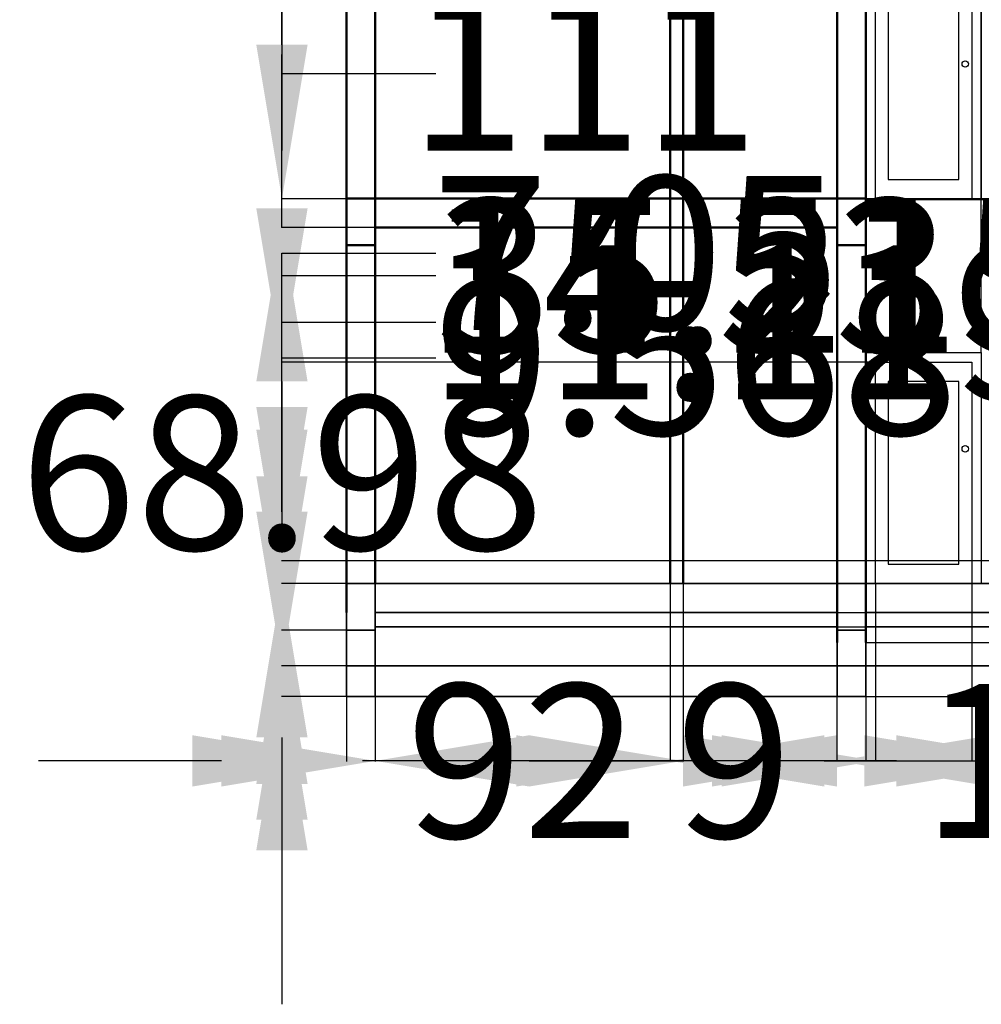
# Model space of a CAD drawing. Units: inches. Extents: x 131 to 858, y -65 to 554.
# Tile 1 of 4: x 131 to 431, y -65 to 242. Entities that reach past the tile are written whole.
import ezdxf

# ---------------------------------------------------------------- set-up
doc = ezdxf.new("R2010")
doc.units = ezdxf.units.IN
doc.header["$MEASUREMENT"] = 0
for name, color, linetype, lineweight in [('A-ANNO-DIMS', 2, 'Continuous', 18), ('A-DOOR', 4, 'Continuous', 25), ('A-SECT', 7, 'Continuous', 50), ('S-FNDN', 1, 'Continuous', 35)]:
    doc.layers.add(name, color=color, linetype=linetype, lineweight=lineweight)
doc.styles.get("Standard").update_dxf_attribs({"font": 'arial.ttf'})
doc.dimstyles.get("Standard").update_dxf_attribs({"dimtxt": 48, "dimasz": 48, "dimexe": 0.18, "dimexo": 0.0625, "dimgap": 0.09, "dimtad": 0, "dimtih": 1, "dimtoh": 1, "dimdec": 0, "dimrnd": 72, "dimzin": 0, "dimdsep": 46, "dimlunit": 3, "dimtxsty": 'Standard', "dimcen": 0.09, "dimadec": 0, "dimazin": 0, "dimtfac": 1, "dimtdec": 0, "dimtofl": 0, "dimtmove": 0, "dimatfit": 3, "dimfxl": 1, "dimtolj": 1, "dimtzin": 0, "dimarcsym": 0})

# ---------------------------------------------------------------- blocks, each defined once
blk = doc.blocks.new('*U3')
blk.add_lwpolyline([(3.12, 0.01), (0.12, 0.01), (0.12, 72.01), (36.12, 72.01), (36.12, 0.01), (33.12, 0.01)])
for points in [[(33.12, 68.99), (33.12, 0.01), (3.12, 0.01), (3.12, 68.99)], [(29.12, 6.01), (29.12, 62.99), (7.12, 62.99), (7.12, 6.01)]]:
    blk.add_lwpolyline(points, close=True)
blk.add_circle((31.12, 42.01), 1)
blk = doc.blocks.new('*D6')
at = {"layer": 'A-ANNO-DIMS', "color": 0, "lineweight": -2, "transparency": 16777216}
for p, q in [((242.01, 177.49), (242.01, 11.06)), ((233.01, 171.97), (233.01, 11.06)), ((185.01, 11.24), (137.01, 11.24)), ((290.01, 11.24), (338.01, 11.24))]:
    blk.add_line(p, q, dxfattribs=at)
at = {"layer": 'A-ANNO-DIMS', "color": 0, "transparency": 16777216}
for points in [[(185.01, 19.24), (185.01, 3.24), (233.01, 11.24)], [(290.01, 19.24), (290.01, 3.24), (242.01, 11.24)]]:
    blk.add_solid(points, dxfattribs=at)
at = {"layer": 'Defpoints', "color": 0, "transparency": 16777216}
for p in [(242.01, 177.55), (233.01, 172.03), (242.01, 11.24)]:
    blk.add_point(p, dxfattribs=at)
at = {"layer": 'A-ANNO-DIMS', "color": 0, "transparency": 16777216, "insert": (353.89, 11.24), "char_height": 48, "attachment_point": 5}
blk.add_mtext('\\A1;9', dxfattribs=at)
blk = doc.blocks.new('*D7')
at = {"layer": 'A-ANNO-DIMS', "color": 0, "lineweight": -2, "transparency": 16777216}
for p, q in [((334.014446, 66.488918), (334.014446, 11.056024)), ((242.014446, 31.273524), (242.014446, 11.056024)), ((194.014446, 11.236024), (146.014446, 11.236024)), ((382.014446, 11.236024), (430.014446, 11.236024))]:
    blk.add_line(p, q, dxfattribs=at)
at = {"layer": 'A-ANNO-DIMS', "color": 0, "transparency": 16777216}
for points in [[(194.014446, 19.236024), (194.014446, 3.236024), (242.014446, 11.236024)], [(382.014446, 19.236024), (382.014446, 3.236024), (334.014446, 11.236024)]]:
    blk.add_solid(points, dxfattribs=at)
at = {"layer": 'Defpoints', "color": 0, "transparency": 16777216}
for p in [(334.014446, 66.551418), (242.014446, 31.336024), (334.014446, 11.236024)]:
    blk.add_point(p, dxfattribs=at)
at = {"layer": 'A-ANNO-DIMS', "color": 0, "transparency": 16777216, "insert": (288.014446, 11.236024), "char_height": 48, "attachment_point": 5}
blk.add_mtext('\\A1;92', dxfattribs=at)
blk = doc.blocks.new('*D8')
at = {"layer": 'A-ANNO-DIMS', "color": 0, "lineweight": -2, "transparency": 16777216}
for p, q in [((334.01, 66.49), (334.01, 11.06)), ((338.01, 66.49), (338.01, 11.06)), ((286.01, 11.24), (238.01, 11.24)), ((386.01, 11.24), (434.01, 11.24))]:
    blk.add_line(p, q, dxfattribs=at)
at = {"layer": 'A-ANNO-DIMS', "color": 0, "transparency": 16777216}
for points in [[(286.01, 19.24), (286.01, 3.24), (334.01, 11.24)], [(386.01, 19.24), (386.01, 3.24), (338.01, 11.24)]]:
    blk.add_solid(points, dxfattribs=at)
at = {"layer": 'Defpoints', "color": 0, "transparency": 16777216}
for p in [(334.01, 66.55), (338.01, 66.55), (338.01, 11.24)]:
    blk.add_point(p, dxfattribs=at)
at = {"layer": 'A-ANNO-DIMS', "color": 0, "transparency": 16777216, "insert": (450.7, 11.24), "char_height": 48, "attachment_point": 5}
blk.add_mtext('\\A1;4', dxfattribs=at)
blk = doc.blocks.new('*D9')
at = {"layer": 'A-ANNO-DIMS', "color": 0, "lineweight": -2, "transparency": 16777216}
for p, q in [((338.01, 66.49), (338.01, 11.06)), ((386.01, 31.27), (386.01, 11.06)), ((290.01, 11.24), (242.01, 11.24)), ((434.01, 11.24), (482.01, 11.24))]:
    blk.add_line(p, q, dxfattribs=at)
at = {"layer": 'A-ANNO-DIMS', "color": 0, "transparency": 16777216}
for points in [[(290.01, 19.24), (290.01, 3.24), (338.01, 11.24)], [(434.01, 19.24), (434.01, 3.24), (386.01, 11.24)]]:
    blk.add_solid(points, dxfattribs=at)
at = {"layer": 'Defpoints', "color": 0, "transparency": 16777216}
for p in [(338.01, 66.55), (386.01, 31.34), (386.01, 11.24)]:
    blk.add_point(p, dxfattribs=at)
at = {"layer": 'A-ANNO-DIMS', "color": 0, "transparency": 16777216, "insert": (517.5, 11.24), "char_height": 48, "attachment_point": 5}
blk.add_mtext('\\A1;48', dxfattribs=at)
blk = doc.blocks.new('*D10')
at = {"layer": 'A-ANNO-DIMS', "color": 0, "lineweight": -2, "transparency": 16777216}
for p, q in [((386.01, 31.27), (386.01, 11.06)), ((395.01, 31.27), (395.01, 11.06)), ((338.01, 11.24), (290.01, 11.24)), ((443.01, 11.24), (491.01, 11.24))]:
    blk.add_line(p, q, dxfattribs=at)
at = {"layer": 'A-ANNO-DIMS', "color": 0, "transparency": 16777216}
for points in [[(338.01, 19.24), (338.01, 3.24), (386.01, 11.24)], [(443.01, 19.24), (443.01, 3.24), (395.01, 11.24)]]:
    blk.add_solid(points, dxfattribs=at)
at = {"layer": 'Defpoints', "color": 0, "transparency": 16777216}
for p in [(386.01, 31.34), (395.01, 31.34), (395.01, 11.24)]:
    blk.add_point(p, dxfattribs=at)
at = {"layer": 'A-ANNO-DIMS', "color": 0, "transparency": 16777216, "insert": (506.89, 11.24), "char_height": 48, "attachment_point": 5}
blk.add_mtext('\\A1;9', dxfattribs=at)
blk = doc.blocks.new('*D11')
at = {"layer": 'A-ANNO-DIMS', "color": 0, "lineweight": -2, "transparency": 16777216}
for p, q in [((395.014446, 31.273524), (395.014446, 11.056024)), ((539.014446, 31.273524), (539.014446, 11.056024)), ((347.014446, 11.236024), (299.014446, 11.236024)), ((587.014446, 11.236024), (635.014446, 11.236024))]:
    blk.add_line(p, q, dxfattribs=at)
at = {"layer": 'A-ANNO-DIMS', "color": 0, "transparency": 16777216}
for points in [[(347.014446, 19.236024), (347.014446, 3.236024), (395.014446, 11.236024)], [(587.014446, 19.236024), (587.014446, 3.236024), (539.014446, 11.236024)]]:
    blk.add_solid(points, dxfattribs=at)
at = {"layer": 'Defpoints', "color": 0, "transparency": 16777216}
for p in [(395.014446, 31.336024), (539.014446, 31.336024), (539.014446, 11.236024)]:
    blk.add_point(p, dxfattribs=at)
at = {"layer": 'A-ANNO-DIMS', "color": 0, "transparency": 16777216, "insert": (467.014446, 11.236024), "char_height": 48, "attachment_point": 5}
blk.add_mtext('\\A1;144', dxfattribs=at)
blk = doc.blocks.new('*D14')
at = {"layer": 'A-ANNO-DIMS', "color": 0, "lineweight": -2, "transparency": 16777216}
for p, q in [((592.11, 426.55), (612.82, 426.55)), ((612.64, 378.55), (612.64, 253.56)), ((612.64, 79.34), (612.64, 204.33)), ((233.08, 31.34), (612.82, 31.34))]:
    blk.add_line(p, q, dxfattribs=at)
at = {"layer": 'A-ANNO-DIMS', "color": 0, "transparency": 16777216}
for points in [[(604.64, 378.55), (620.64, 378.55), (612.64, 426.55)], [(604.64, 79.34), (620.64, 79.34), (612.64, 31.34)]]:
    blk.add_solid(points, dxfattribs=at)
at = {"layer": 'Defpoints', "color": 0, "transparency": 16777216}
for p in [(592.04, 426.55), (612.64, 426.55), (233.01, 31.34)]:
    blk.add_point(p, dxfattribs=at)
at = {"layer": 'A-ANNO-DIMS', "color": 0, "transparency": 16777216, "insert": (612.64, 228.94), "char_height": 48, "attachment_point": 5}
blk.add_mtext('\\A1;395.2', dxfattribs=at)
blk = doc.blocks.new('*D15')
at = {"layer": 'A-ANNO-DIMS', "color": 0, "lineweight": -2, "transparency": 16777216}
for p, q in [((212.91, 114.55), (212.91, 162.55)), ((212.91, 162.55), (260.91, 162.55)), ((385.95, 66.55), (212.73, 66.55)), ((385.95, 31.34), (212.73, 31.34)), ((212.91, -16.66), (212.91, -64.66))]:
    blk.add_line(p, q, dxfattribs=at)
at = {"layer": 'A-ANNO-DIMS', "color": 0, "transparency": 16777216}
for points in [[(204.91, 114.55), (220.91, 114.55), (212.91, 66.55)], [(204.91, -16.66), (220.91, -16.66), (212.91, 31.34)]]:
    blk.add_solid(points, dxfattribs=at)
at = {"layer": 'Defpoints', "color": 0, "transparency": 16777216}
for p in [(212.91, 66.55), (386.01, 66.55), (386.01, 31.34)]:
    blk.add_point(p, dxfattribs=at)
at = {"layer": 'A-ANNO-DIMS', "color": 0, "transparency": 16777216, "insert": (360.8, 162.55), "char_height": 48, "attachment_point": 5}
blk.add_mtext('\\A1;35.215', dxfattribs=at)
blk = doc.blocks.new('*D16')
at = {"layer": 'A-ANNO-DIMS', "color": 0, "lineweight": -2, "transparency": 16777216}
for p, q in [((212.91, 88.9), (212.91, 136.9)), ((212.91, 136.9), (260.91, 136.9)), ((232.95, 40.9), (212.73, 40.9)), ((232.95, 31.34), (212.73, 31.34)), ((212.91, -16.66), (212.91, -64.66))]:
    blk.add_line(p, q, dxfattribs=at)
at = {"layer": 'A-ANNO-DIMS', "color": 0, "transparency": 16777216}
for points in [[(204.91, 88.9), (220.91, 88.9), (212.91, 40.9)], [(204.91, -16.66), (220.91, -16.66), (212.91, 31.34)]]:
    blk.add_solid(points, dxfattribs=at)
at = {"layer": 'Defpoints', "color": 0, "transparency": 16777216}
for p in [(212.91, 40.9), (233.01, 40.9), (233.01, 31.34)]:
    blk.add_point(p, dxfattribs=at)
at = {"layer": 'A-ANNO-DIMS', "color": 0, "transparency": 16777216, "insert": (342.04, 136.9), "char_height": 48, "attachment_point": 5}
blk.add_mtext('\\A1;9.568', dxfattribs=at)
blk = doc.blocks.new('*D17')
at = {"layer": 'A-ANNO-DIMS', "color": 0, "lineweight": -2, "transparency": 16777216}
for p, q in [((212.91, 100.02), (212.91, 148.02)), ((212.91, 148.02), (260.91, 148.02)), ((232.95, 52.02), (212.73, 52.02)), ((232.95, 40.9), (212.73, 40.9)), ((212.91, -7.1), (212.91, -55.1))]:
    blk.add_line(p, q, dxfattribs=at)
at = {"layer": 'A-ANNO-DIMS', "color": 0, "transparency": 16777216}
for points in [[(204.91, 100.02), (220.91, 100.02), (212.91, 52.02)], [(204.91, -7.1), (220.91, -7.1), (212.91, 40.9)]]:
    blk.add_solid(points, dxfattribs=at)
at = {"layer": 'Defpoints', "color": 0, "transparency": 16777216}
for p in [(212.91, 52.02), (233.01, 52.02), (233.01, 40.9)]:
    blk.add_point(p, dxfattribs=at)
at = {"layer": 'A-ANNO-DIMS', "color": 0, "transparency": 16777216, "insert": (358.43, 148.02), "char_height": 48, "attachment_point": 5}
blk.add_mtext('\\A1;11.119', dxfattribs=at)
blk = doc.blocks.new('*D18')
at = {"layer": 'A-ANNO-DIMS', "color": 0, "lineweight": -2, "transparency": 16777216}
for p, q in [((212.91, 114.55), (212.91, 162.55)), ((212.91, 162.55), (260.91, 162.55)), ((232.95, 66.55), (212.73, 66.55)), ((232.95, 52.02), (212.73, 52.02)), ((212.91, 4.02), (212.91, -43.98))]:
    blk.add_line(p, q, dxfattribs=at)
at = {"layer": 'A-ANNO-DIMS', "color": 0, "transparency": 16777216}
for points in [[(204.91, 114.55), (220.91, 114.55), (212.91, 66.55)], [(204.91, 4.02), (220.91, 4.02), (212.91, 52.02)]]:
    blk.add_solid(points, dxfattribs=at)
at = {"layer": 'Defpoints', "color": 0, "transparency": 16777216}
for p in [(212.91, 66.55), (233.01, 66.55), (233.01, 52.02)]:
    blk.add_point(p, dxfattribs=at)
at = {"layer": 'A-ANNO-DIMS', "color": 0, "transparency": 16777216, "insert": (339.73, 162.55), "char_height": 48, "attachment_point": 5}
blk.add_mtext('\\A1;14.53', dxfattribs=at)
blk = doc.blocks.new('*D19')
at = {"layer": 'A-ANNO-DIMS', "color": 0, "lineweight": -2, "transparency": 16777216}
for p, q in [((612.64, 105.55), (612.64, 153.55)), ((612.64, 153.55), (660.64, 153.55)), ((242.08, 57.55), (612.82, 57.55)), ((242.08, 53.09), (612.82, 53.09)), ((612.64, 5.09), (612.64, -42.91))]:
    blk.add_line(p, q, dxfattribs=at)
at = {"layer": 'A-ANNO-DIMS', "color": 0, "transparency": 16777216}
for points in [[(604.64, 105.55), (620.64, 105.55), (612.64, 57.55)], [(604.64, 5.09), (620.64, 5.09), (612.64, 53.09)]]:
    blk.add_solid(points, dxfattribs=at)
at = {"layer": 'Defpoints', "color": 0, "transparency": 16777216}
for p in [(242.01, 57.55), (612.64, 57.55), (242.01, 53.09)]:
    blk.add_point(p, dxfattribs=at)
at = {"layer": 'A-ANNO-DIMS', "color": 0, "transparency": 16777216, "insert": (742.86, 153.55), "char_height": 48, "attachment_point": 5}
blk.add_mtext('\\A1;4.465', dxfattribs=at)
blk = doc.blocks.new('*D20')
at = {"layer": 'A-ANNO-DIMS', "color": 0, "lineweight": -2, "transparency": 16777216}
for p, q in [((612.64, 114.55), (612.64, 162.55)), ((612.64, 162.55), (660.64, 162.55)), ((242.08, 66.55), (612.82, 66.55)), ((242.08, 57.55), (612.82, 57.55)), ((612.64, 9.55), (612.64, -38.45))]:
    blk.add_line(p, q, dxfattribs=at)
at = {"layer": 'A-ANNO-DIMS', "color": 0, "transparency": 16777216}
for points in [[(604.64, 114.55), (620.64, 114.55), (612.64, 66.55)], [(604.64, 9.55), (620.64, 9.55), (612.64, 57.55)]]:
    blk.add_solid(points, dxfattribs=at)
at = {"layer": 'Defpoints', "color": 0, "transparency": 16777216}
for p in [(242.01, 66.55), (612.64, 66.55), (242.01, 57.55)]:
    blk.add_point(p, dxfattribs=at)
at = {"layer": 'A-ANNO-DIMS', "color": 0, "transparency": 16777216, "insert": (676.51, 162.55), "char_height": 48, "attachment_point": 5}
blk.add_mtext('\\A1;9', dxfattribs=at)
blk = doc.blocks.new('*D21')
at = {"layer": 'A-ANNO-DIMS', "color": 0, "lineweight": -2, "transparency": 16777216}
for p, q in [((233.01, 31.27), (233.01, 11.06)), ((242.01, 31.27), (242.01, 11.06)), ((185.01, 11.24), (137.01, 11.24)), ((290.01, 11.24), (338.01, 11.24))]:
    blk.add_line(p, q, dxfattribs=at)
at = {"layer": 'A-ANNO-DIMS', "color": 0, "transparency": 16777216}
for points in [[(185.01, 19.24), (185.01, 3.24), (233.01, 11.24)], [(290.01, 19.24), (290.01, 3.24), (242.01, 11.24)]]:
    blk.add_solid(points, dxfattribs=at)
at = {"layer": 'Defpoints', "color": 0, "transparency": 16777216}
for p in [(233.01, 31.34), (242.01, 31.34), (242.01, 11.24)]:
    blk.add_point(p, dxfattribs=at)
at = {"layer": 'A-ANNO-DIMS', "color": 0, "transparency": 16777216, "insert": (353.89, 11.24), "char_height": 48, "attachment_point": 5}
blk.add_mtext('\\A1;9', dxfattribs=at)
blk = doc.blocks.new('*D22')
at = {"layer": 'A-ANNO-DIMS', "color": 0, "lineweight": -2, "transparency": 16777216}
for p, q in [((612.64, 114.55), (612.64, 162.55)), ((612.64, 162.55), (660.64, 162.55)), ((395.08, 66.55), (612.82, 66.55)), ((395.08, 48.13), (612.82, 48.13)), ((612.64, 0.13), (612.64, -47.87))]:
    blk.add_line(p, q, dxfattribs=at)
at = {"layer": 'A-ANNO-DIMS', "color": 0, "transparency": 16777216}
for points in [[(604.64, 114.55), (620.64, 114.55), (612.64, 66.55)], [(604.64, 0.13), (620.64, 0.13), (612.64, 48.13)]]:
    blk.add_solid(points, dxfattribs=at)
at = {"layer": 'Defpoints', "color": 0, "transparency": 16777216}
for p in [(395.01, 66.55), (612.64, 66.55), (395.01, 48.13)]:
    blk.add_point(p, dxfattribs=at)
at = {"layer": 'A-ANNO-DIMS', "color": 0, "transparency": 16777216, "insert": (758.11, 162.55), "char_height": 48, "attachment_point": 5}
blk.add_mtext('\\A1;18.417', dxfattribs=at)
blk = doc.blocks.new('*D23')
at = {"layer": 'A-ANNO-DIMS', "color": 0, "lineweight": -2, "transparency": 16777216}
for p, q in [((212.91, 177.55), (212.91, 225.55)), ((212.91, 225.55), (260.91, 225.55)), ((241.95, 177.55), (212.73, 177.55)), ((212.91, 114.55), (212.91, 129.55)), ((232.95, 66.55), (212.73, 66.55))]:
    blk.add_line(p, q, dxfattribs=at)
at = {"layer": 'A-ANNO-DIMS', "color": 0, "transparency": 16777216}
for points in [[(204.91, 129.55), (220.91, 129.55), (212.91, 177.55)], [(204.91, 114.55), (220.91, 114.55), (212.91, 66.55)]]:
    blk.add_solid(points, dxfattribs=at)
at = {"layer": 'Defpoints', "color": 0, "transparency": 16777216}
for p in [(212.91, 177.55), (242.01, 177.55), (233.01, 66.55)]:
    blk.add_point(p, dxfattribs=at)
at = {"layer": 'A-ANNO-DIMS', "color": 0, "transparency": 16777216, "insert": (307.14, 225.55), "char_height": 48, "attachment_point": 5}
blk.add_mtext('\\A1;111', dxfattribs=at)
blk = doc.blocks.new('*D24')
at = {"layer": 'A-ANNO-DIMS', "color": 0, "lineweight": -2, "transparency": 16777216}
for p, q in [((212.91, 234.55), (212.91, 282.55)), ((212.91, 282.55), (260.91, 282.55)), ((232.95, 186.55), (212.73, 186.55)), ((241.95, 177.55), (212.73, 177.55)), ((212.91, 129.55), (212.91, 81.55))]:
    blk.add_line(p, q, dxfattribs=at)
at = {"layer": 'A-ANNO-DIMS', "color": 0, "transparency": 16777216}
for points in [[(204.91, 234.55), (220.91, 234.55), (212.91, 186.55)], [(204.91, 129.55), (220.91, 129.55), (212.91, 177.55)]]:
    blk.add_solid(points, dxfattribs=at)
at = {"layer": 'Defpoints', "color": 0, "transparency": 16777216}
for p in [(212.91, 186.55), (233.01, 186.55), (242.01, 177.55)]:
    blk.add_point(p, dxfattribs=at)
at = {"layer": 'A-ANNO-DIMS', "color": 0, "transparency": 16777216, "insert": (276.79, 282.55), "char_height": 48, "attachment_point": 5}
blk.add_mtext('\\A1;9', dxfattribs=at)
blk = doc.blocks.new('*D25')
at = {"layer": 'A-ANNO-DIMS', "color": 0, "lineweight": -2, "transparency": 16777216}
for p, q in [((212.91, 297.55), (212.91, 345.55)), ((212.91, 345.55), (260.91, 345.55)), ((241.95, 297.55), (212.73, 297.55)), ((212.91, 234.55), (212.91, 249.55)), ((232.95, 186.55), (212.73, 186.55))]:
    blk.add_line(p, q, dxfattribs=at)
at = {"layer": 'A-ANNO-DIMS', "color": 0, "transparency": 16777216}
for points in [[(204.91, 249.55), (220.91, 249.55), (212.91, 297.55)], [(204.91, 234.55), (220.91, 234.55), (212.91, 186.55)]]:
    blk.add_solid(points, dxfattribs=at)
at = {"layer": 'Defpoints', "color": 0, "transparency": 16777216}
for p in [(212.91, 297.55), (242.01, 297.55), (233.01, 186.55)]:
    blk.add_point(p, dxfattribs=at)
at = {"layer": 'A-ANNO-DIMS', "color": 0, "transparency": 16777216, "insert": (307.14, 345.55), "char_height": 48, "attachment_point": 5}
blk.add_mtext('\\A1;111', dxfattribs=at)
blk = doc.blocks.new('*D26')
at = {"layer": 'A-ANNO-DIMS', "color": 0, "lineweight": -2, "transparency": 16777216}
for p, q in [((212.91, 354.55), (212.91, 402.55)), ((212.91, 402.55), (260.91, 402.55)), ((232.95, 306.55), (212.73, 306.55)), ((241.95, 297.55), (212.73, 297.55)), ((212.91, 249.55), (212.91, 201.55))]:
    blk.add_line(p, q, dxfattribs=at)
at = {"layer": 'A-ANNO-DIMS', "color": 0, "transparency": 16777216}
for points in [[(204.91, 354.55), (220.91, 354.55), (212.91, 306.55)], [(204.91, 249.55), (220.91, 249.55), (212.91, 297.55)]]:
    blk.add_solid(points, dxfattribs=at)
at = {"layer": 'Defpoints', "color": 0, "transparency": 16777216}
for p in [(212.91, 306.55), (233.01, 306.55), (242.01, 297.55)]:
    blk.add_point(p, dxfattribs=at)
at = {"layer": 'A-ANNO-DIMS', "color": 0, "transparency": 16777216, "insert": (276.79, 402.55), "char_height": 48, "attachment_point": 5}
blk.add_mtext('\\A1;9', dxfattribs=at)
blk = doc.blocks.new('*D27')
at = {"layer": 'A-ANNO-DIMS', "color": 0, "lineweight": -2, "transparency": 16777216}
for p, q in [((212.91, 402.55), (212.91, 450.55)), ((212.91, 450.55), (260.91, 450.55)), ((232.95, 354.55), (212.73, 354.55)), ((232.95, 306.55), (212.73, 306.55)), ((212.91, 258.55), (212.91, 210.55))]:
    blk.add_line(p, q, dxfattribs=at)
at = {"layer": 'A-ANNO-DIMS', "color": 0, "transparency": 16777216}
for points in [[(204.91, 402.55), (220.91, 402.55), (212.91, 354.55)], [(204.91, 258.55), (220.91, 258.55), (212.91, 306.55)]]:
    blk.add_solid(points, dxfattribs=at)
at = {"layer": 'Defpoints', "color": 0, "transparency": 16777216}
for p in [(212.91, 354.55), (233.01, 354.55), (233.01, 306.55)]:
    blk.add_point(p, dxfattribs=at)
at = {"layer": 'A-ANNO-DIMS', "color": 0, "transparency": 16777216, "insert": (296.4, 450.55), "char_height": 48, "attachment_point": 5}
blk.add_mtext('\\A1;48', dxfattribs=at)
blk = doc.blocks.new('*D32')
at = {"layer": 'A-ANNO-DIMS', "color": 0, "lineweight": -2, "transparency": 16777216}
for p, q in [((347.01, 446.65), (299.01, 446.65)), ((395.01, 138.61), (395.01, 446.83)), ((431.01, 138.61), (431.01, 446.83)), ((479.01, 446.65), (527.01, 446.65))]:
    blk.add_line(p, q, dxfattribs=at)
at = {"layer": 'A-ANNO-DIMS', "color": 0, "transparency": 16777216}
for points in [[(347.01, 454.65), (347.01, 438.65), (395.01, 446.65)], [(479.01, 454.65), (479.01, 438.65), (431.01, 446.65)]]:
    blk.add_solid(points, dxfattribs=at)
at = {"layer": 'Defpoints', "color": 0, "transparency": 16777216}
for p in [(431.01, 446.65), (395.01, 138.55), (431.01, 138.55)]:
    blk.add_point(p, dxfattribs=at)
at = {"layer": 'A-ANNO-DIMS', "color": 0, "transparency": 16777216, "insert": (561.45, 446.65), "char_height": 48, "attachment_point": 5}
blk.add_mtext('\\A1;36', dxfattribs=at)
blk = doc.blocks.new('*D34')
at = {"layer": 'A-ANNO-DIMS', "color": 0, "lineweight": -2, "transparency": 16777216}
for p, q in [((398.01, 66.49), (398.01, 11.06)), ((428.01, 66.49), (428.01, 11.06)), ((350.01, 11.24), (302.01, 11.24)), ((476.01, 11.24), (524.01, 11.24))]:
    blk.add_line(p, q, dxfattribs=at)
at = {"layer": 'A-ANNO-DIMS', "color": 0, "transparency": 16777216}
for points in [[(350.01, 19.24), (350.01, 3.24), (398.01, 11.24)], [(476.01, 19.24), (476.01, 3.24), (428.01, 11.24)]]:
    blk.add_solid(points, dxfattribs=at)
at = {"layer": 'Defpoints', "color": 0, "transparency": 16777216}
for p in [(398.01, 66.55), (428.01, 66.55), (428.01, 11.24)]:
    blk.add_point(p, dxfattribs=at)
at = {"layer": 'A-ANNO-DIMS', "color": 0, "transparency": 16777216, "insert": (558.39, 11.24), "char_height": 48, "attachment_point": 5}
blk.add_mtext('\\A1;30', dxfattribs=at)
blk = doc.blocks.new('*D35')
at = {"layer": 'A-ANNO-DIMS', "color": 0, "lineweight": -2, "transparency": 16777216}
for p, q in [((212.91, 183.53), (212.91, 231.53)), ((397.95, 135.53), (212.73, 135.53)), ((397.95, 66.55), (212.73, 66.55)), ((212.91, 18.55), (212.91, -29.45))]:
    blk.add_line(p, q, dxfattribs=at)
at = {"layer": 'A-ANNO-DIMS', "color": 0, "transparency": 16777216}
for points in [[(204.91, 183.53), (220.91, 183.53), (212.91, 135.53)], [(204.91, 18.55), (220.91, 18.55), (212.91, 66.55)]]:
    blk.add_solid(points, dxfattribs=at)
at = {"layer": 'Defpoints', "color": 0, "transparency": 16777216}
for p in [(212.91, 135.53), (398.01, 135.53), (398.01, 66.55)]:
    blk.add_point(p, dxfattribs=at)
at = {"layer": 'A-ANNO-DIMS', "color": 0, "transparency": 16777216, "insert": (212.91, 101.04), "char_height": 48, "attachment_point": 5}
blk.add_mtext('\\A1;68.98', dxfattribs=at)
blk = doc.blocks.new('*D36')
at = {"layer": 'A-ANNO-DIMS', "color": 0, "lineweight": -2, "transparency": 16777216}
for p, q in [((452.53, 73.54), (452.53, 11.06)), ((442.52, 66.49), (442.52, 11.06)), ((394.52, 11.24), (346.52, 11.24)), ((500.53, 11.24), (548.53, 11.24))]:
    blk.add_line(p, q, dxfattribs=at)
at = {"layer": 'A-ANNO-DIMS', "color": 0, "transparency": 16777216}
for points in [[(394.52, 19.24), (394.52, 3.24), (442.52, 11.24)], [(500.53, 19.24), (500.53, 3.24), (452.53, 11.24)]]:
    blk.add_solid(points, dxfattribs=at)
at = {"layer": 'Defpoints', "color": 0, "transparency": 16777216}
for p in [(452.53, 73.6), (442.52, 66.55), (452.53, 11.24)]:
    blk.add_point(p, dxfattribs=at)
at = {"layer": 'A-ANNO-DIMS', "color": 0, "transparency": 16777216, "insert": (646, 11.24), "char_height": 48, "attachment_point": 5}
blk.add_mtext('\\A1;10.013', dxfattribs=at)
blk = doc.blocks.new('*D37')
at = {"layer": 'A-ANNO-DIMS', "color": 0, "lineweight": -2, "transparency": 16777216}
for p, q in [((544.04, 126.29), (544.04, 11.06)), ((452.53, 73.54), (452.53, 11.06)), ((404.53, 11.24), (356.53, 11.24)), ((592.04, 11.24), (640.04, 11.24))]:
    blk.add_line(p, q, dxfattribs=at)
at = {"layer": 'A-ANNO-DIMS', "color": 0, "transparency": 16777216}
for points in [[(404.53, 19.24), (404.53, 3.24), (452.53, 11.24)], [(592.04, 19.24), (592.04, 3.24), (544.04, 11.24)]]:
    blk.add_solid(points, dxfattribs=at)
at = {"layer": 'Defpoints', "color": 0, "transparency": 16777216}
for p in [(544.04, 126.36), (452.53, 73.6), (544.04, 11.24)]:
    blk.add_point(p, dxfattribs=at)
at = {"layer": 'A-ANNO-DIMS', "color": 0, "transparency": 16777216, "insert": (716.49, 11.24), "char_height": 48, "attachment_point": 5}
blk.add_mtext('\\A1;91.51', dxfattribs=at)
blk = doc.blocks.new('*D40')
at = {"layer": 'A-ANNO-DIMS', "color": 0, "lineweight": -2, "transparency": 16777216}
for p, q in [((212.91, 121.6), (212.91, 169.6)), ((212.91, 169.6), (260.91, 169.6)), ((442.46, 73.6), (212.73, 73.6)), ((442.46, 66.55), (212.73, 66.55)), ((212.91, 18.55), (212.91, -29.45))]:
    blk.add_line(p, q, dxfattribs=at)
at = {"layer": 'A-ANNO-DIMS', "color": 0, "transparency": 16777216}
for points in [[(204.91, 121.6), (220.91, 121.6), (212.91, 73.6)], [(204.91, 18.55), (220.91, 18.55), (212.91, 66.55)]]:
    blk.add_solid(points, dxfattribs=at)
at = {"layer": 'Defpoints', "color": 0, "transparency": 16777216}
for p in [(212.91, 73.6), (442.52, 73.6), (442.52, 66.55)]:
    blk.add_point(p, dxfattribs=at)
at = {"layer": 'A-ANNO-DIMS', "color": 0, "transparency": 16777216, "insert": (323.33, 169.6), "char_height": 48, "attachment_point": 5}
blk.add_mtext('\\A1;7.05', dxfattribs=at)

msp = doc.modelspace()

# ---------------------------------------------------------------- linework, layer by layer
at = {"layer": 'A-SECT'}
for p, q in [((395.0144, 48.1342), (395.0144, 366.3568)), ((386.0144, 48.1342), (386.0144, 354.5514)), ((233.0144, 306.5514), (233.0144, 57.5514)), ((242.0144, 306.5514), (242.0144, 66.5514)), ((334.0144, 306.5514), (334.0144, 66.5514)), ((338.0144, 306.5514), (338.0144, 66.5514)), ((386.0144, 306.5514), (386.0144, 66.5514)), ((395.0144, 306.5514), (395.0144, 57.5514)), ((233.0144, 172.0345), (233.0144, 186.5514)), ((233.0144, 186.5514), (242.0144, 186.5514)), ((242.0144, 186.5514), (386.0144, 186.5514)), ((242.0144, 186.5514), (386.0144, 186.5514)), ((242.0144, 186.5514), (242.0144, 177.5514)), ((386.0144, 172.0345), (386.0144, 186.5514)), ((386.0144, 186.5514), (395.0144, 186.5514)), ((395.0144, 186.5514), (395.0144, 177.5514)), ((395.0144, 186.3568), (443.0144, 186.3568)), ((395.0144, 186.3568), (395.0144, 48.1342)), ((242.0144, 177.5514), (386.0144, 177.5514)), ((242.0144, 172.0345), (233.0144, 172.0345)), ((395.0144, 172.0345), (386.0144, 172.0345))]:
    msp.add_line(p, q, dxfattribs=at)
at = {"layer": 'S-FNDN'}
for p, q in [((242.0144, 66.5514), (233.0144, 66.5514)), ((242.0144, 66.5514), (386.0144, 66.5514)), ((242.0144, 66.5514), (242.0144, 57.5514)), ((386.0144, 66.5514), (395.0144, 66.5514)), ((395.0144, 66.5514), (386.0144, 66.5514)), ((386.0144, 66.5514), (386.0144, 57.5514)), ((395.0144, 66.5514), (386.0144, 66.5514)), ((442.5179, 66.5514), (386.0144, 66.5514)), ((395.0144, 66.5514), (548.0144, 66.5514)), ((395.0144, 66.5514), (395.0144, 57.5514)), ((233.0144, 31.336), (233.0144, 57.5514)), ((242.0144, 57.5514), (386.0144, 57.5514)), ((242.0144, 57.5514), (242.0144, 31.336)), ((386.0144, 31.336), (386.0144, 57.5514)), ((395.0144, 57.5514), (539.0144, 57.5514)), ((395.0144, 57.5514), (395.0144, 31.336)), ((242.0144, 53.0868), (386.0144, 53.0868)), ((395.0144, 53.0868), (539.0144, 53.0868)), ((233.0144, 52.0226), (242.0144, 52.0226)), ((386.0144, 52.0226), (395.0144, 52.0226)), ((386.0144, 52.0226), (395.0144, 52.0226)), ((233.0144, 40.9038), (548.0144, 40.9038)), ((233.0144, 31.336), (242.0144, 31.336)), ((386.0144, 31.336), (395.0144, 31.336))]:
    msp.add_line(p, q, dxfattribs=at)

# ---------------------------------------------------------------- block references
at = {"layer": 'A-DOOR'}
for p in [(394.8907, 186.5387), (394.8907, 66.5387)]:
    msp.add_blockref('*U3', p, dxfattribs=at)

# ---------------------------------------------------------------- dimensions: what is measured, and where the dimension line sits
at = {"layer": 'A-ANNO-DIMS'}
for base, p1, p2, override, picture, middle in [((212.9144, 354.5514), (233.0144, 306.5514), (233.0144, 354.5514), {"dimdec": 0, "dimlfac": 1, "dimrnd": 0, "dimzin": 0, "dimdsep": 46, "dimlunit": 2}, '*D27', (296.3987, 450.5514)), ((212.9144, 306.5514), (242.0144, 297.5514), (233.0144, 306.5514), {"dimdec": 0, "dimlfac": 1, "dimrnd": 0, "dimzin": 0, "dimdsep": 46, "dimlunit": 2}, '*D26', (276.7862, 402.5514)), ((612.64, 426.5514), (233.0144, 31.336), (592.0434, 426.5514), {"dimdec": 1, "dimlfac": 1, "dimrnd": 0, "dimzin": 0, "dimdsep": 46, "dimlunit": 2}, '*D14', (612.64, 228.9437)), ((212.9144, 297.5514), (233.0144, 186.5514), (242.0144, 297.5514), {"dimdec": 0, "dimlfac": 1, "dimrnd": 0, "dimzin": 0, "dimdsep": 46, "dimlunit": 2}, '*D25', (307.1381, 345.5514)), ((212.9144, 186.5514), (242.0144, 177.5514), (233.0144, 186.5514), {"dimdec": 0, "dimlfac": 1, "dimrnd": 0, "dimzin": 0, "dimdsep": 46, "dimlunit": 2}, '*D24', (276.7862, 282.5514)), ((212.9144, 177.5514), (233.0144, 66.5514), (242.0144, 177.5514), {"dimdec": 0, "dimlfac": 1, "dimrnd": 0, "dimzin": 0, "dimdsep": 46, "dimlunit": 2}, '*D23', (307.1381, 225.5514)), ((212.9144, 135.5284), (398.0144, 66.5514), (398.0144, 135.5284), {"dimdec": 2, "dimlfac": 1, "dimrnd": 0, "dimzin": 0, "dimdsep": 46, "dimlunit": 2}, '*D35', (212.9144, 101.0399)), ((212.9144, 73.6016), (442.5179, 66.5514), (442.5179, 73.6016), {"dimdec": 2, "dimlfac": 1, "dimrnd": 0, "dimzin": 0, "dimdsep": 46, "dimlunit": 2}, '*D40', (323.3291, 169.6016)), ((212.9144, 66.5514), (386.0144, 31.336), (386.0144, 66.5514), {"dimdec": 3, "dimlfac": 1, "dimrnd": 0, "dimzin": 0, "dimdsep": 46, "dimlunit": 2}, '*D15', (360.8025, 162.5514)), ((212.9144, 66.5514), (233.0144, 52.0226), (233.0144, 66.5514), {"dimdec": 2, "dimlfac": 1, "dimrnd": 0, "dimzin": 0, "dimdsep": 46, "dimlunit": 2}, '*D18', (339.733, 162.5514)), ((612.64, 66.5514), (242.0144, 57.5514), (242.0144, 66.5514), {"dimdec": 0, "dimlfac": 1, "dimrnd": 0, "dimzin": 0, "dimdsep": 46, "dimlunit": 2}, '*D20', (676.5117, 162.5514)), ((612.64, 66.5514), (395.0144, 48.1342), (395.0144, 66.5514), {"dimdec": 3, "dimlfac": 1, "dimrnd": 0, "dimzin": 0, "dimdsep": 46, "dimlunit": 2}, '*D22', (758.1051, 162.5514)), ((612.64, 57.5514), (242.0144, 53.0868), (242.0144, 57.5514), {"dimdec": 3, "dimlfac": 1, "dimrnd": 0, "dimzin": 0, "dimdsep": 46, "dimlunit": 2}, '*D19', (742.8637, 153.5514)), ((212.9144, 52.0226), (233.0144, 40.9038), (233.0144, 52.0226), {"dimdec": 3, "dimlfac": 1, "dimrnd": 0, "dimzin": 0, "dimdsep": 46, "dimlunit": 2}, '*D17', (358.4287, 148.0226)), ((212.9144, 40.9038), (233.0144, 31.336), (233.0144, 40.9038), {"dimdec": 3, "dimlfac": 1, "dimrnd": 0, "dimzin": 0, "dimdsep": 46, "dimlunit": 2}, '*D16', (342.0413, 136.9038))]:
    dim = msp.add_linear_dim(base=base, p1=p1, p2=p2, angle=90, dimstyle='Standard', override=override, dxfattribs=at)
    dim.commit()
    dim.dimension.update_dxf_attribs({"geometry": picture, "text_midpoint": middle})
for base, p1, p2, override, picture, middle in [((431.0144, 446.6514), (395.0144, 138.5514), (431.0144, 138.5514), {"dimdec": 0, "dimlfac": 1, "dimrnd": 0, "dimzin": 0, "dimdsep": 46, "dimlunit": 2}, '*D32', (561.451, 446.6514)), ((242.0144, 11.236), (233.0144, 172.0345), (242.0144, 177.5514), {"dimdec": 0, "dimlfac": 1, "dimrnd": 0, "dimzin": 0, "dimdsep": 46, "dimlunit": 2}, '*D6', (353.8862, 11.236)), ((544.0434, 11.236), (452.5306, 73.6016), (544.0434, 126.3568), {"dimdec": 2, "dimlfac": 1, "dimrnd": 0, "dimzin": 0, "dimdsep": 46, "dimlunit": 2}, '*D37', (716.4881, 11.236)), ((452.5306, 11.236), (442.5179, 66.5514), (452.5306, 73.6016), {"dimdec": 3, "dimlfac": 1, "dimrnd": 0, "dimzin": 0, "dimdsep": 46, "dimlunit": 2}, '*D36', (645.9958, 11.236)), ((334.0144, 11.236), (242.0144, 31.336), (334.0144, 66.5514), {"dimdec": 0, "dimlfac": 1, "dimrnd": 0, "dimzin": 0, "dimdsep": 46, "dimlunit": 2}, '*D7', (288.0144, 11.236)), ((338.0144, 11.236), (334.0144, 66.5514), (338.0144, 66.5514), {"dimdec": 0, "dimlfac": 1, "dimrnd": 0, "dimzin": 0, "dimdsep": 46, "dimlunit": 2}, '*D8', (450.7047, 11.236)), ((386.0144, 11.236), (338.0144, 66.5514), (386.0144, 31.336), {"dimdec": 0, "dimlfac": 1, "dimrnd": 0, "dimzin": 0, "dimdsep": 46, "dimlunit": 2}, '*D9', (517.4987, 11.236)), ((428.0144, 11.236), (398.0144, 66.5514), (428.0144, 66.5514), {"dimdec": 0, "dimlfac": 1, "dimrnd": 0, "dimzin": 0, "dimdsep": 46, "dimlunit": 2}, '*D34', (558.3855, 11.236)), ((242.0144, 11.236), (233.0144, 31.336), (242.0144, 31.336), {"dimdec": 0, "dimlfac": 1, "dimrnd": 0, "dimzin": 0, "dimdsep": 46, "dimlunit": 2}, '*D21', (353.8862, 11.236)), ((395.0144, 11.236), (386.0144, 31.336), (395.0144, 31.336), {"dimdec": 0, "dimlfac": 1, "dimrnd": 0, "dimzin": 0, "dimdsep": 46, "dimlunit": 2}, '*D10', (506.8862, 11.236)), ((539.0144, 11.236), (395.0144, 31.336), (539.0144, 31.336), {"dimdec": 0, "dimlfac": 1, "dimrnd": 0, "dimzin": 0, "dimdsep": 46, "dimlunit": 2}, '*D11', (467.0144, 11.236))]:
    dim = msp.add_linear_dim(base=base, p1=p1, p2=p2, dimstyle='Standard', override=override, dxfattribs=at)
    dim.commit()
    dim.dimension.update_dxf_attribs({"geometry": picture, "text_midpoint": middle})

doc.saveas('drawing.dxf')
